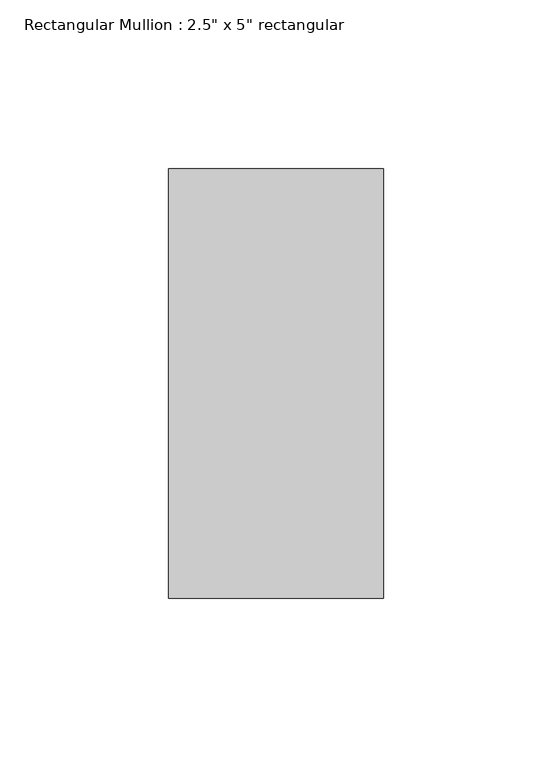
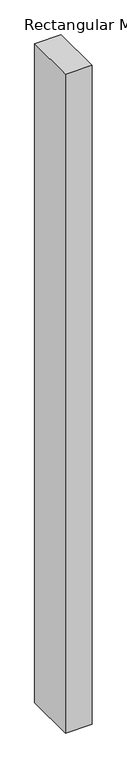
"""IFC4 building model written with IfcOpenShell, lengths in millimetres: member geometry."""

from ifc_helpers import new_model, si_unit, frame, origin, place, context, project, spatial, polyline, outline, extrude, source, transform, mapped, element, save


def member_d9b49a07(model_context):
    return source(origin(), model_context, "Body", "SweptSolid", [
        extrude(outline(polyline([(0.0, 63.5), (0.0, -63.5), (-63.5, -63.5), (-63.5, 63.5), (0.0, 63.5)])), frame((0.0, 0.0, -1663.8745067), z_axis=(0.0, 0.0, 1.0), x_axis=(1.0, 0.0, 0.0)), (0.0, 0.0, 1.0), 1663.8745067),
    ])


if __name__ == "__main__":
    model = new_model("IFC4")
    model_context = context("Model", 3, world=origin())
    ifc_project = project(units=[si_unit("LENGTHUNIT", "METRE", prefix="MILLI")], contexts=[model_context])
    site = spatial("IfcSite", under=ifc_project)
    building = spatial("IfcBuilding", under=site)
    placement = place(None, origin())
    member_shape = member_d9b49a07(model_context)
    element("IfcMember", 1, ObjectType="Rectangular Mullion : 2.5\" x 5\" rectangular", at=placement, inside=building, context=model_context, shape_type="MappedRepresentation", body=[
        mapped(member_shape, transform((0.0, 0.0, 0.0), x_axis=(1.0, 0.0, 0.0), y_axis=(0.0, 1.0, 0.0), z_axis=(0.0, 0.0, 1.0))),
    ])
    save(model, "model.ifc")

# Revit data of these elements
# Type "Rectangular Mullion : 2.5\" x 5\" rectangular"
#   built-in parameter 1007304 = 0.416667 (stored number, unit not read)
#   built-in parameter 1007301 = 0.104167 (stored number, unit not read)
#   built-in parameter 1007300 = 0.104167 (stored number, unit not read)
# Element 1 (IfcMember, "Rectangular Mullion : 2.5\" x 5\" rectangular")
#   Materials on its faces: "Aluminum"
# Materials
#   "Aluminum": class "Metal", colour RGB 247 247 247, transparency 0, Description = "Aluminum 6061", Cost = 0
